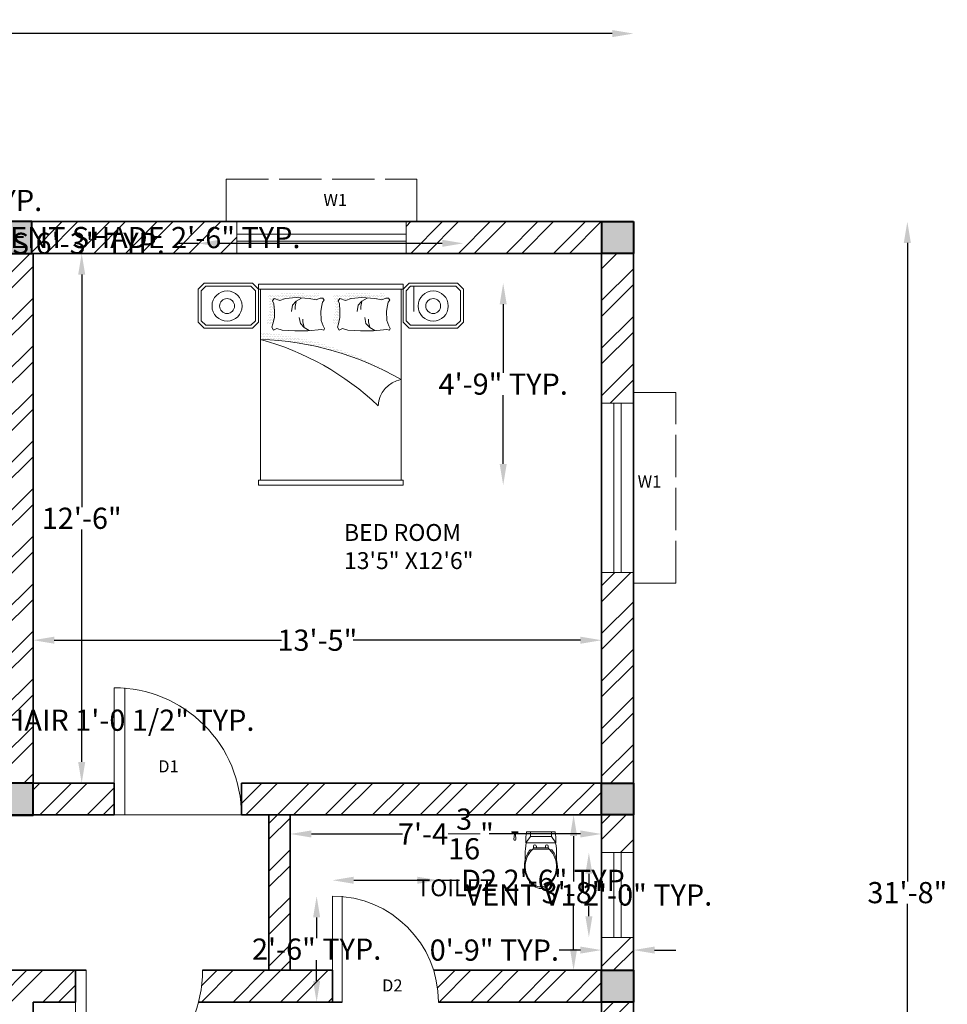
# Model space of a CAD drawing. Units: inches. Extents: x 3614 to 4242, y 2406 to 3033.
# Tile 10 of 10: x 3980 to 4242, y 2733 to 3012. Entities that reach past the tile are written whole.
import ezdxf

# ---------------------------------------------------------------- set-up
doc = ezdxf.new("R2010")
doc.units = ezdxf.units.IN
doc.linetypes.add('ACAD_ISO02W100', pattern=[15, 12, -3])
for name, color, linetype, lineweight in [('A-ANNO-DIMS', 2, 'Continuous', 18), ('A-ANNO-TEXT', 7, 'Continuous', 18), ('A-AREA-IDEN', 7, 'Continuous', 25), ('A-COLS', 7, 'Continuous', 40), ('A-COLS-PATT', 252, 'Continuous', 18), ('A-DOOR', 3, 'Continuous', 18), ('A-FLOR-FIXT', 9, 'Continuous', 18), ('A-FURN', 8, 'Continuous', 18), ('A-GLAZ', 4, 'Continuous', 18), ('A-GLAZ-OVHD', 8, 'ACAD_ISO02W100', 13), ('A-WALL', 7, 'Continuous', 35), ('A-WALL-PATT', 252, 'Continuous', 13)]:
    doc.layers.add(name, color=color, linetype=linetype, lineweight=lineweight)
doc.styles.get("Standard").update_dxf_attribs({"font": 'arial.ttf'})
doc.dimstyles.get("Standard").update_dxf_attribs({"dimtxt": 6, "dimasz": 6, "dimexe": 0.18, "dimexo": 0.0625, "dimgap": 0.09, "dimtad": 0, "dimtih": 1, "dimtoh": 1, "dimdec": 4, "dimzin": 0, "dimdsep": 46, "dimlunit": 4, "dimtxsty": 'Standard', "dimcen": 0.09, "dimse1": 1, "dimse2": 1, "dimadec": 0, "dimazin": 0, "dimtfac": 1, "dimtdec": 4, "dimtofl": 0, "dimtmove": 0, "dimatfit": 3, "dimfxl": 1, "dimtolj": 1, "dimtzin": 0, "dimarcsym": 0})
pattern_1 = [(270, (-3578.6833, 5895.14276), (0.451673685, -0.225836843), [0, -0.451673685])]

# ---------------------------------------------------------------- blocks, each defined once
blk = doc.blocks.new('*D8')
at = {"layer": 'A-ANNO-DIMS', "color": 0, "lineweight": -2, "transparency": 16777216}
for p, q in [((4136.4, 2780.34), (4136.4, 2767.5)), ((4136.4, 2748.34), (4136.4, 2761.19))]:
    blk.add_line(p, q, dxfattribs=at)
at = {"layer": 'A-ANNO-DIMS', "color": 0, "transparency": 16777216}
for points in [[(4135.4, 2780.34), (4137.4, 2780.34), (4136.4, 2786.34)], [(4135.4, 2748.34), (4137.4, 2748.34), (4136.4, 2742.34)]]:
    blk.add_solid(points, dxfattribs=at)
at = {"layer": 'Defpoints', "color": 0, "transparency": 16777216}
for p in [(4144.34, 2786.34), (4136.4, 2742.34), (4144.34, 2742.34)]:
    blk.add_point(p, dxfattribs=at)
at = {"layer": 'A-ANNO-DIMS', "color": 0, "transparency": 16777216, "insert": (4136.4, 2764.34), "char_height": 6, "attachment_point": 5}
blk.add_mtext('\\A1;3\'-8"', dxfattribs=at)
blk = doc.blocks.new('*D9')
at = {"layer": 'A-ANNO-DIMS', "color": 0, "lineweight": -2, "transparency": 16777216}
for p, q in [((4062.14, 2780.95), (4087.99, 2780.95)), ((4138.34, 2780.95), (4112.49, 2780.95))]:
    blk.add_line(p, q, dxfattribs=at)
at = {"layer": 'A-ANNO-DIMS', "color": 0, "transparency": 16777216}
for points in [[(4062.14, 2781.95), (4062.14, 2779.95), (4056.14, 2780.95)], [(4138.34, 2781.95), (4138.34, 2779.95), (4144.34, 2780.95)]]:
    blk.add_solid(points, dxfattribs=at)
at = {"layer": 'Defpoints', "color": 0, "transparency": 16777216}
for p in [(4056.14, 2786.34), (4144.34, 2786.34), (4144.34, 2780.95)]:
    blk.add_point(p, dxfattribs=at)
at = {"layer": 'A-ANNO-DIMS', "color": 0, "transparency": 16777216, "insert": (4100.24, 2780.95), "char_height": 6, "attachment_point": 5}
blk.add_mtext('\\A1;7\'-4{\\H1x;\\S3/16;}"', dxfattribs=at)
blk = doc.blocks.new('*D21')
at = {"layer": 'A-ANNO-DIMS', "color": 0, "lineweight": -2, "transparency": 16777216}
for p, q in [((3997.11, 2939.34), (3997.11, 2873.49)), ((3997.11, 2801.34), (3997.11, 2867.19))]:
    blk.add_line(p, q, dxfattribs=at)
at = {"layer": 'A-ANNO-DIMS', "color": 0, "transparency": 16777216}
for points in [[(3996.11, 2939.34), (3998.11, 2939.34), (3997.11, 2945.34)], [(3996.11, 2801.34), (3998.11, 2801.34), (3997.11, 2795.34)]]:
    blk.add_solid(points, dxfattribs=at)
at = {"layer": 'Defpoints', "color": 0, "transparency": 16777216}
for p in [(3992.71, 2945.34), (3992.71, 2795.34), (3997.11, 2795.34)]:
    blk.add_point(p, dxfattribs=at)
at = {"layer": 'A-ANNO-DIMS', "color": 0, "transparency": 16777216, "insert": (3997.11, 2870.34), "char_height": 6, "attachment_point": 5}
blk.add_mtext('\\A1;12\'-6"', dxfattribs=at)
blk = doc.blocks.new('*D22')
at = {"layer": 'A-ANNO-DIMS', "color": 0, "lineweight": -2, "transparency": 16777216}
for p, q in [((3989.34, 2835.82), (4053.72, 2835.82)), ((4138.34, 2835.82), (4073.95, 2835.82))]:
    blk.add_line(p, q, dxfattribs=at)
at = {"layer": 'A-ANNO-DIMS', "color": 0, "transparency": 16777216}
for points in [[(3989.34, 2836.82), (3989.34, 2834.82), (3983.34, 2835.82)], [(4138.34, 2836.82), (4138.34, 2834.82), (4144.34, 2835.82)]]:
    blk.add_solid(points, dxfattribs=at)
at = {"layer": 'Defpoints', "color": 0, "transparency": 16777216}
for p in [(3983.34, 2843.38), (4144.34, 2843.38), (4144.34, 2835.82)]:
    blk.add_point(p, dxfattribs=at)
at = {"layer": 'A-ANNO-DIMS', "color": 0, "transparency": 16777216, "insert": (4063.84, 2835.82), "char_height": 6, "attachment_point": 5}
blk.add_mtext('\\A1;13\'-5"', dxfattribs=at)
blk = doc.blocks.new('*D24')
at = {"layer": 'A-ANNO-DIMS', "color": 0, "lineweight": -2, "transparency": 16777216}
for p, q in [((3694.34, 3007.6), (3910.44, 3007.6)), ((4147.34, 3007.6), (3931.23, 3007.6))]:
    blk.add_line(p, q, dxfattribs=at)
at = {"layer": 'A-ANNO-DIMS', "color": 0, "transparency": 16777216}
for points in [[(3694.34, 3008.6), (3694.34, 3006.6), (3688.34, 3007.6)], [(4147.34, 3008.6), (4147.34, 3006.6), (4153.34, 3007.6)]]:
    blk.add_solid(points, dxfattribs=at)
at = {"layer": 'Defpoints', "color": 0, "transparency": 16777216}
for p in [(4153.34, 3007.6), (3688.34, 2954.34), (4153.34, 2954.34)]:
    blk.add_point(p, dxfattribs=at)
at = {"layer": 'A-ANNO-DIMS', "color": 0, "transparency": 16777216, "insert": (3920.84, 3007.6), "char_height": 6, "attachment_point": 5}
blk.add_mtext('\\A1;38\'-9"', dxfattribs=at)
blk = doc.blocks.new('*D25')
at = {"layer": 'A-ANNO-DIMS', "color": 0, "lineweight": -2, "transparency": 16777216}
for p, q in [((4230.92, 2948.34), (4230.92, 2767.5)), ((4230.92, 2580.34), (4230.92, 2761.19))]:
    blk.add_line(p, q, dxfattribs=at)
at = {"layer": 'A-ANNO-DIMS', "color": 0, "transparency": 16777216}
for points in [[(4229.92, 2948.34), (4231.92, 2948.34), (4230.92, 2954.34)], [(4229.92, 2580.34), (4231.92, 2580.34), (4230.92, 2574.34)]]:
    blk.add_solid(points, dxfattribs=at)
at = {"layer": 'Defpoints', "color": 0, "transparency": 16777216}
for p in [(4153.34, 2954.34), (4153.34, 2574.34), (4230.92, 2574.34)]:
    blk.add_point(p, dxfattribs=at)
at = {"layer": 'A-ANNO-DIMS', "color": 0, "transparency": 16777216, "insert": (4230.92, 2764.34), "char_height": 6, "attachment_point": 5}
blk.add_mtext('\\A1;31\'-8"', dxfattribs=at)
blk = doc.blocks.new('WINDOW-W1-48IN')
for p, q in [((48, 9), (0, 9)), ((0, 9), (0, 0)), ((48, 0), (48, 9)), ((0, 5.5), (48, 5.5)), ((0, 3.5), (48, 3.5)), ((0, 0), (48, 0))]:
    blk.add_line(p, q)
blk = doc.blocks.new('VENT-V1-24IN')
for p, q in [((24, 9), (0, 9)), ((0, 9), (0, 0)), ((24, 0), (24, 9)), ((0, 5.5), (24, 5.5)), ((0, 3.5), (24, 3.5)), ((0, 0), (24, 0))]:
    blk.add_line(p, q)
blk = doc.blocks.new('SHADE-W1')
for p, q in [((0, 0), (0, 12)), ((0, 12), (51, 12)), ((51, 12), (54, 12)), ((54, 12), (54, 0)), ((3, 0), (0, 0))]:
    blk.add_line(p, q)
blk = doc.blocks.new('COLUMN-9X9')
blk.add_lwpolyline([(9, 9), (0, 9), (0, 0), (9, 0)], close=True)
blk = doc.blocks.new('DOOR-SWING-30IN')
for p, q in [((0, 30), (0, 0)), ((2.75, 30), (2.75, 0)), ((0, 0), (2.75, 0))]:
    blk.add_line(p, q)
blk.add_arc((0, 0), 30, 0, 90)
blk = doc.blocks.new('DOOR-SWING-36IN')
for p, q in [((0, 36), (0, 0)), ((0, 0), (0, 36)), ((3, 0), (3, 36))]:
    blk.add_line(p, q)
blk.add_arc((0, 36), 36, 270, 0)
blk = doc.blocks.new('WC-PLAN')
for p, q in [((5.97, 11.16), (6.2, 11.58)), ((6.2, 11.58), (6.2, 12.03)), ((7.01, 11.58), (6.2, 11.58)), ((7.01, 12.03), (7.01, 11.58)), ((8.3, 11.58), (7.01, 11.58)), ((8.3, 11.58), (9.59, 11.58)), ((9.59, 12.03), (9.59, 11.58)), ((9.59, 11.58), (10.39, 11.58)), ((10.39, 11.58), (10.39, 12.03)), ((10.62, 11.16), (10.39, 11.58))]:
    blk.add_line(p, q)
for points in [[(1.85, 16.08), (0, 16.08)], [(1.73, 15.95), (0.11, 15.95)], [(1.35, 15.74), (0.5, 15.74)], [(0.5, 15.74), (0.5, 15.47), (0.8, 15.47)], [(0.72, 15.74), (0.72, 15.47)], [(0.8, 15.47), (1.07, 15.47)], [(1.07, 15.47), (1.34, 15.47), (1.35, 15.74)], [(1.15, 15.74), (1.15, 15.47)], [(4.05, 12.98), (5.32, 14.75), (5.32, 16.08)], [(12.37, 16.08), (4.22, 16.08)], [(5.32, 14.75), (8.3, 14.75)], [(11.28, 14.75), (8.3, 14.75)], [(12.54, 12.98), (11.28, 14.75), (11.28, 16.08)], [(4.13, 12.98), (8.3, 12.98)], [(12.47, 12.98), (8.3, 12.98)]]:
    blk.add_lwpolyline(points)
for points in [[(0.5, 15.74, -0.158381), (0, 16.08, 2.932383)], [(0.8, 15.45), (0.63, 13.98, 0.482607), (0.95, 13.67, -0.547905)], [(1.07, 15.45), (1.23, 13.98, -0.482607), (0.92, 13.67, 0.547905)], [(1.35, 15.74, 0.158381), (1.85, 16.08, -2.932383)], [(4.22, 16.08, 0.056711), (4.05, 12.98), (4.13, 12.98)], [(12.37, 16.08, -0.056711), (12.54, 12.98), (12.47, 12.98)], [(4.13, 12.98, 0.052121), (3.84, 9.61), (3.84, 8.13, 0.14456)], [(5.97, 11.16, 0.008985), (5.8, 11, 0.182634)], [(8.3, 11.16), (5.97, 11.16, 0.008985)], [(8.3, 11.16), (10.62, 11.16, -0.444938)], [(10.62, 11.16, -0.008985), (10.79, 11, -0.182634)], [(12.47, 12.98, -0.052121), (12.76, 9.61), (12.76, 8.13, -0.14456)], [(5.24, 11, 0.11024), (3.84, 8.13, 0.16845)], [(5.8, 11, 0.434217), (6.2, 1.23, 0.182634), (8.3, 0.47, 2.693815)], [(5.8, 11), (5.24, 11, 0.416606)], [(10.79, 11, -0.434217), (10.39, 1.23, -0.182634), (8.3, 0.47, -2.693815)], [(10.79, 11), (11.35, 11, -0.416606)], [(11.35, 11, -0.11024), (12.76, 8.13, -0.16845)], [(3.84, 8.13, 0.292914), (6.42, 0.65, 0.16845), (8.3, 0, 2.883082)], [(12.76, 8.13, -0.292914), (10.17, 0.65, -0.16845), (8.3, 0, -2.883082)]]:
    blk.add_lwpolyline(points, format="xyb")
for centre in [(6.6, 12.03), (9.99, 12.03)]:
    blk.add_arc(centre, 0.403, 0, 180)
blk = doc.blocks.new('BED-DOUBLE-WITH-NIGHTSTANDS')
h = blk.add_hatch()
h.set_pattern_fill('DOTS', color=256, scale=0.284519, angle=-90, style=0)
h.set_pattern_definition(pattern_1)
h.paths.add_polyline_path([(43.21, 57.47), (41.26, 57.47, -0.124273), (29.87, 17.64, 0.122563)])
h = blk.add_hatch()
h.set_pattern_fill('DOTS', color=256, scale=0.284519, angle=-90, style=0)
h.set_pattern_definition(pattern_1)
h.paths.add_polyline_path([(53.82, 40.86), (54.34, 41.21), (54.34, 42), (53.9, 43.14), (54.25, 45.06), (54.52, 48.74), (54.25, 51.8), (53.73, 53.38), (54.25, 55.04), (53.55, 55.48), (52.77, 55.13), (50.75, 54.95), (48.83, 54.95), (47.08, 55.39), (46.12, 55.65), (45.33, 55.22), (45.77, 54.25), (45.69, 53.96), (47.41, 53.53), (49.34, 53.53), (51.35, 53.71), (52.13, 54.06), (52.83, 53.62), (52.31, 51.96), (52.83, 50.38), (53.1, 47.32), (52.83, 43.64), (52.48, 41.72), (52.6, 41.41), (53.2, 41.3)])
h.paths.add_polyline_path([(53.82, 22.27), (54.34, 22.62), (54.34, 23.41), (53.9, 24.55), (54.25, 26.48), (54.52, 30.15), (54.25, 33.21), (53.73, 34.79), (54.25, 36.45), (53.55, 36.89), (52.77, 36.54), (50.75, 36.37), (48.83, 36.37), (47.08, 36.8), (46.12, 37.07), (45.33, 36.63), (45.77, 35.67), (45.69, 35.38), (47.41, 34.95), (49.34, 34.95), (51.35, 35.12), (52.13, 35.47), (52.83, 35.03), (52.31, 33.37), (52.83, 31.79), (53.1, 28.73), (52.83, 25.05), (52.48, 23.13), (52.6, 22.82), (53.2, 22.71)])
for p, q in [((0, 17.07), (0, 58.04)), ((0, 58.04), (1.42, 58.04)), ((1.42, 17.07), (1.42, 58.04)), ((1.42, 57.47), (55.48, 57.47)), ((55.48, 17.07), (55.48, 58.04)), ((55.48, 58.04), (56.9, 58.04)), ((56.9, 17.07), (56.9, 58.04)), ((1.42, 17.07), (0, 17.07)), ((55.48, 17.64), (1.42, 17.64)), ((56.9, 17.07), (55.48, 17.07)), ((56.3, 14.01), (49.19, 14.01))]:
    blk.add_line(p, q)
for points in [[(44.39, 73.41), (44.39, 59.75), (46.09, 58.04), (55.48, 58.04), (57.19, 59.75), (57.19, 73.41), (55.48, 75.11), (46.09, 75.11)], [(45.24, 72.98), (45.24, 60.18), (46.52, 58.9), (55.05, 58.9), (56.33, 60.18), (56.33, 72.98), (55.05, 74.26), (46.52, 74.26)], [(44.39, 15.36), (44.39, 1.71), (46.09, 0), (55.48, 0), (57.19, 1.71), (57.19, 15.36), (55.48, 17.07), (46.09, 17.07)], [(45.24, 14.94), (45.24, 2.13), (46.52, 0.85), (55.05, 0.85), (56.33, 2.13), (56.33, 14.94), (55.05, 16.22), (46.52, 16.22)]]:
    blk.add_lwpolyline(points, close=True)
for points in [[(52.31, 51.96), (52.83, 53.62), (52.13, 54.06), (51.35, 53.71), (49.34, 53.53), (47.41, 53.53), (45.66, 53.97), (44.7, 54.23), (43.91, 53.8), (44.35, 52.83), (43.91, 51.34), (43.65, 47.76), (43.65, 44.08), (44.09, 40.23), (43.91, 39.53), (44.35, 39.35), (45.05, 39.7), (46.62, 40.32), (49.25, 40.4), (50.82, 40.05), (51.78, 39.88), (52.4, 39.44), (52.92, 39.79), (52.92, 40.58), (52.48, 41.72), (52.83, 43.64), (53.1, 47.32), (52.83, 50.38), (52.31, 51.96)], [(52.92, 45.83), (52.05, 47.32), (50.91, 48.37), (49.16, 48.72)], [(51.96, 47.32), (50.56, 47.67), (49.69, 47.67)], [(43.74, 43.64), (44.61, 45.13), (45.75, 46.18), (47.5, 46.53)], [(44.7, 45.13), (46.1, 45.48), (46.97, 45.48)], [(52.31, 33.37), (52.83, 35.03), (52.13, 35.47), (51.35, 35.12), (49.34, 34.95), (47.41, 34.95), (45.66, 35.38), (44.7, 35.65), (43.91, 35.21), (44.35, 34.24), (43.91, 32.76), (43.65, 29.17), (43.65, 25.49), (44.09, 21.64), (43.91, 20.94), (44.35, 20.77), (45.05, 21.12), (46.62, 21.73), (49.25, 21.82), (50.82, 21.47), (51.78, 21.29), (52.4, 20.85), (52.92, 21.2), (52.92, 21.99), (52.48, 23.13), (52.83, 25.05), (53.1, 28.73), (52.83, 31.79), (52.31, 33.37)], [(43.74, 25.05), (44.61, 26.54), (45.75, 27.59), (47.5, 27.94)], [(52.92, 27.24), (52.05, 28.73), (50.91, 29.78), (49.16, 30.13)], [(51.96, 28.73), (50.56, 29.08), (49.69, 29.08)], [(44.7, 26.54), (46.1, 26.89), (46.97, 26.89)]]:
    blk.add_lwpolyline(points)
for centre, radius in [((50.7, 66.92), 4.27), ((50.7, 66.92), 2.11), ((50.7, 8.56), 4.27), ((50.7, 8.56), 2.11)]:
    blk.add_circle(centre, radius)
for centre, radius, start, end in [((-34.21, 78.09), 78.23, 316.4367, 344.7234), ((-43.33, 60.1), 84.62, 329.8866, 358.2226), ((22.03, 16.21), 7.98, 10.3543, 86.7862)]:
    blk.add_arc(centre, radius, start, end)
blk = doc.blocks.new('*D45')
at = {"layer": 'A-ANNO-DIMS', "color": 0, "lineweight": -2, "transparency": 16777216}
for p, q in [((3931.73, 2825.5), (3931.73, 2825.16)), ((3931.73, 2819.16), (3931.73, 2813.16)), ((3931.73, 2813.16), (3937.73, 2813.16))]:
    blk.add_line(p, q, dxfattribs=at)
at = {"layer": 'A-ANNO-DIMS', "color": 0, "transparency": 16777216}
for points in [[(3932.73, 2825.5), (3930.73, 2825.5), (3931.73, 2831.5)], [(3932.73, 2825.16), (3930.73, 2825.16), (3931.73, 2819.16)]]:
    blk.add_solid(points, dxfattribs=at)
at = {"layer": 'Defpoints', "color": 0, "transparency": 16777216}
for p in [(3933.58, 2831.5), (3931.73, 2819.16), (3933.58, 2819.16)]:
    blk.add_point(p, dxfattribs=at)
at = {"layer": 'A-ANNO-DIMS', "color": 0, "transparency": 16777216, "insert": (3992.99, 2813.16), "char_height": 6, "attachment_point": 5}
blk.add_mtext('\\A1;DINING CHAIR 1\'-0 1/2" TYP.', dxfattribs=at)
blk = doc.blocks.new('*D47')
at = {"layer": 'A-ANNO-DIMS', "color": 0, "lineweight": -2, "transparency": 16777216}
for p, q in [((4140.74, 2769.67), (4140.74, 2766.82)), ((4140.74, 2757.67), (4140.74, 2760.51))]:
    blk.add_line(p, q, dxfattribs=at)
at = {"layer": 'A-ANNO-DIMS', "color": 0, "transparency": 16777216}
for points in [[(4139.74, 2769.67), (4141.74, 2769.67), (4140.74, 2775.67)], [(4139.74, 2757.67), (4141.74, 2757.67), (4140.74, 2751.67)]]:
    blk.add_solid(points, dxfattribs=at)
at = {"layer": 'Defpoints', "color": 0, "transparency": 16777216}
for p in [(4140.74, 2775.67), (4144.34, 2775.67), (4144.34, 2751.67)]:
    blk.add_point(p, dxfattribs=at)
at = {"layer": 'A-ANNO-DIMS', "color": 0, "transparency": 16777216, "insert": (4140.74, 2763.67), "char_height": 6, "attachment_point": 5}
blk.add_mtext('\\A1;VENT V1 2\'-0" TYP.', dxfattribs=at)
blk = doc.blocks.new('*D48')
at = {"layer": 'A-ANNO-DIMS', "color": 0, "lineweight": -2, "transparency": 16777216}
for p, q in [((4138.34, 2748.07), (4132.34, 2748.07)), ((4159.34, 2748.07), (4165.34, 2748.07))]:
    blk.add_line(p, q, dxfattribs=at)
at = {"layer": 'A-ANNO-DIMS', "color": 0, "transparency": 16777216}
for points in [[(4138.34, 2749.07), (4138.34, 2747.07), (4144.34, 2748.07)], [(4159.34, 2749.07), (4159.34, 2747.07), (4153.34, 2748.07)]]:
    blk.add_solid(points, dxfattribs=at)
at = {"layer": 'Defpoints', "color": 0, "transparency": 16777216}
for p in [(4144.34, 2751.67), (4153.34, 2751.67), (4144.34, 2748.07)]:
    blk.add_point(p, dxfattribs=at)
at = {"layer": 'A-ANNO-DIMS', "color": 0, "transparency": 16777216, "insert": (4113.96, 2748.07), "char_height": 6, "attachment_point": 5}
blk.add_mtext('\\A1;0\'-9" TYP.', dxfattribs=at)
blk = doc.blocks.new('*D51')
at = {"layer": 'A-ANNO-DIMS', "color": 0, "lineweight": -2, "transparency": 16777216}
for p, q in [((3939.12, 2949.84), (3957.12, 2949.84)), ((3963.12, 2949.84), (3969.12, 2949.84))]:
    blk.add_line(p, q, dxfattribs=at)
at = {"layer": 'A-ANNO-DIMS', "color": 0, "transparency": 16777216}
for points in [[(3939.12, 2950.84), (3939.12, 2948.84), (3933.12, 2949.84)], [(3957.12, 2950.84), (3957.12, 2948.84), (3963.12, 2949.84)]]:
    blk.add_solid(points, dxfattribs=at)
at = {"layer": 'Defpoints', "color": 0, "transparency": 16777216}
for p in [(3933.12, 2954.34), (3963.12, 2954.34), (3963.12, 2949.84)]:
    blk.add_point(p, dxfattribs=at)
at = {"layer": 'A-ANNO-DIMS', "color": 0, "transparency": 16777216, "insert": (4015.6, 2949.84), "char_height": 6, "attachment_point": 5}
blk.add_mtext('\\A1;VENT SHADE 2\'-6" TYP.', dxfattribs=at)
blk = doc.blocks.new('*D52')
at = {"layer": 'A-ANNO-DIMS', "color": 0, "lineweight": -2, "transparency": 16777216}
for p, q in [((3967.62, 2972.34), (3967.62, 2978.34)), ((3967.62, 2948.34), (3967.62, 2942.34))]:
    blk.add_line(p, q, dxfattribs=at)
at = {"layer": 'A-ANNO-DIMS', "color": 0, "transparency": 16777216}
for points in [[(3966.62, 2972.34), (3968.62, 2972.34), (3967.62, 2966.34)], [(3966.62, 2948.34), (3968.62, 2948.34), (3967.62, 2954.34)]]:
    blk.add_solid(points, dxfattribs=at)
at = {"layer": 'Defpoints', "color": 0, "transparency": 16777216}
for p in [(3963.12, 2966.34), (3967.62, 2966.34), (3963.12, 2954.34)]:
    blk.add_point(p, dxfattribs=at)
at = {"layer": 'A-ANNO-DIMS', "color": 0, "transparency": 16777216, "insert": (3967.62, 2960.34), "char_height": 6, "attachment_point": 5}
blk.add_mtext('\\A1;1\'-0" TYP.', dxfattribs=at)
blk = doc.blocks.new('*D53')
at = {"layer": 'A-ANNO-DIMS', "color": 0, "lineweight": -2, "transparency": 16777216}
for p, q in [((4074.14, 2767.84), (4092.14, 2767.84)), ((4098.14, 2767.84), (4104.14, 2767.84))]:
    blk.add_line(p, q, dxfattribs=at)
at = {"layer": 'A-ANNO-DIMS', "color": 0, "transparency": 16777216}
for points in [[(4074.14, 2768.84), (4074.14, 2766.84), (4068.14, 2767.84)], [(4092.14, 2768.84), (4092.14, 2766.84), (4098.14, 2767.84)]]:
    blk.add_solid(points, dxfattribs=at)
at = {"layer": 'Defpoints', "color": 0, "transparency": 16777216}
for p in [(4098.14, 2767.84), (4068.14, 2763.34), (4098.14, 2763.34)]:
    blk.add_point(p, dxfattribs=at)
at = {"layer": 'A-ANNO-DIMS', "color": 0, "transparency": 16777216, "insert": (4128.89, 2767.84), "char_height": 6, "attachment_point": 5}
blk.add_mtext('\\A1;D2 2\'-6" TYP.', dxfattribs=at)
blk = doc.blocks.new('*D54')
at = {"layer": 'A-ANNO-DIMS', "color": 0, "lineweight": -2, "transparency": 16777216}
for p, q in [((4063.64, 2757.34), (4063.64, 2751.49)), ((4063.64, 2739.34), (4063.64, 2745.19))]:
    blk.add_line(p, q, dxfattribs=at)
at = {"layer": 'A-ANNO-DIMS', "color": 0, "transparency": 16777216}
for points in [[(4062.64, 2757.34), (4064.64, 2757.34), (4063.64, 2763.34)], [(4062.64, 2739.34), (4064.64, 2739.34), (4063.64, 2733.34)]]:
    blk.add_solid(points, dxfattribs=at)
at = {"layer": 'Defpoints', "color": 0, "transparency": 16777216}
for p in [(4063.64, 2763.34), (4068.14, 2763.34), (4068.14, 2733.34)]:
    blk.add_point(p, dxfattribs=at)
at = {"layer": 'A-ANNO-DIMS', "color": 0, "transparency": 16777216, "insert": (4063.64, 2748.34), "char_height": 6, "attachment_point": 5}
blk.add_mtext('\\A1;2\'-6" TYP.', dxfattribs=at)
blk = doc.blocks.new('*D57')
at = {"layer": 'A-ANNO-DIMS', "color": 0, "lineweight": -2, "transparency": 16777216}
for p, q in [((4030.09, 2948.2), (4024.09, 2948.2)), ((4099.2, 2948.2), (4036.09, 2948.2))]:
    blk.add_line(p, q, dxfattribs=at)
at = {"layer": 'A-ANNO-DIMS', "color": 0, "transparency": 16777216}
for points in [[(4036.09, 2949.2), (4036.09, 2947.2), (4030.09, 2948.2)], [(4099.2, 2949.2), (4099.2, 2947.2), (4105.2, 2948.2)]]:
    blk.add_solid(points, dxfattribs=at)
at = {"layer": 'Defpoints', "color": 0, "transparency": 16777216}
for p in [(4030.09, 2948.2), (4030.09, 2936.94), (4105.2, 2936.94)]:
    blk.add_point(p, dxfattribs=at)
at = {"layer": 'A-ANNO-DIMS', "color": 0, "transparency": 16777216, "insert": (3960.9, 2948.2), "char_height": 6, "attachment_point": 5}
blk.add_mtext('\\A1;BED & NIGHTSTANDS 6\'-3" TYP.', dxfattribs=at)
blk = doc.blocks.new('*D58')
at = {"layer": 'A-ANNO-DIMS', "color": 0, "lineweight": -2, "transparency": 16777216}
for p, q in [((4116.47, 2930.94), (4116.47, 2911.49)), ((4116.47, 2885.75), (4116.47, 2905.19))]:
    blk.add_line(p, q, dxfattribs=at)
at = {"layer": 'A-ANNO-DIMS', "color": 0, "transparency": 16777216}
for points in [[(4115.47, 2930.94), (4117.47, 2930.94), (4116.47, 2936.94)], [(4115.47, 2885.75), (4117.47, 2885.75), (4116.47, 2879.75)]]:
    blk.add_solid(points, dxfattribs=at)
at = {"layer": 'Defpoints', "color": 0, "transparency": 16777216}
for p in [(4105.2, 2936.94), (4116.47, 2936.94), (4105.2, 2879.75)]:
    blk.add_point(p, dxfattribs=at)
at = {"layer": 'A-ANNO-DIMS', "color": 0, "transparency": 16777216, "insert": (4116.47, 2908.34), "char_height": 6, "attachment_point": 5}
blk.add_mtext('\\A1;4\'-9" TYP.', dxfattribs=at)

msp = doc.modelspace()

# ---------------------------------------------------------------- hatches: boundary and pattern name
at = {"layer": 'A-COLS-PATT'}
h = msp.add_hatch(color=256, dxfattribs=at)
h.dxf.hatch_style = 1
h.paths.add_polyline_path([(3697.336, 2954.34049), (3688.336, 2954.34049), (3688.336, 2945.34049), (3697.336, 2945.34049)])
h.paths.add_polyline_path([(3818.336, 2954.34049), (3809.336, 2954.34049), (3809.336, 2945.34049), (3818.336, 2945.34049)])
h.paths.add_polyline_path([(3818.336, 2787.28572), (3809.336, 2787.28572), (3809.336, 2778.34049), (3818.336, 2778.34049)])
h.paths.add_polyline_path([(3697.336, 2742.34049), (3688.336, 2742.34049), (3688.336, 2733.34049), (3697.336, 2733.34049)])
h.paths.add_polyline_path([(3697.336, 2583.37355), (3688.336, 2583.37355), (3688.336, 2574.37355), (3697.336, 2574.37355)])
h.paths.add_polyline_path([(3899.336, 2583.34049), (3890.336, 2583.34049), (3890.336, 2574.34049), (3899.336, 2574.34049)])
h.paths.add_polyline_path([(3983.336, 2583.34049), (3974.336, 2583.34049), (3974.336, 2574.34049), (3983.336, 2574.34049)])
h.paths.add_polyline_path([(4153.336, 2583.34049), (4144.336, 2583.34049), (4144.336, 2574.34049), (4153.336, 2574.34049)])
h.paths.add_polyline_path([(4153.336, 2742.34049), (4144.336, 2742.34049), (4144.336, 2733.34049), (4153.336, 2733.34049)])
h.paths.add_polyline_path([(4153.336, 2795.34049), (4144.336, 2795.34049), (4144.336, 2786.34049), (4153.336, 2786.34049)])
h.paths.add_polyline_path([(3983.336, 2795.31105), (3974.336, 2795.31105), (3974.336, 2786.34049), (3983.336, 2786.34049)])
h.paths.add_polyline_path([(4153.336, 2954.34049), (4144.36882, 2954.34049), (4144.36882, 2945.34049), (4153.336, 2945.34049)])
h.paths.add_polyline_path([(3982.96188, 2954.34049), (3973.96188, 2954.34049), (3973.96188, 2945.34049), (3982.96188, 2945.34049)])
at = {"layer": 'A-WALL-PATT'}
h = msp.add_hatch(dxfattribs=at)
h.set_pattern_fill('ANSI32', color=256)
h.paths.add_polyline_path([(4041.01458, 2954.34049), (3982.96188, 2954.34049), (3982.96188, 2945.34049), (3983.336, 2945.34049), (4041.01458, 2945.34049)])
h.paths.add_polyline_path([(3973.96188, 2954.34049), (3960.11861, 2954.34049), (3960.11861, 2945.34049), (3973.96188, 2945.34049)])
h.paths.add_polyline_path([(3936.11861, 2954.34049), (3901.17016, 2954.34049), (3901.17016, 2945.34049), (3913.336, 2945.34049), (3913.336, 2896.34049, -0.050382044), (3919.336, 2895.73437), (3919.336, 2945.34049), (3936.11861, 2945.34049)])
h.paths.add_polyline_path([(3983.336, 2945.34049), (3982.96188, 2945.34049), (3974.336, 2945.34049), (3974.336, 2873.34049), (3974.336, 2795.31105), (3983.336, 2795.31105), (3983.336, 2867.34049)])
h.paths.add_polyline_path([(3974.336, 2872.34049), (3919.336, 2872.34049), (3858.336, 2872.34049), (3858.336, 2866.34049), (3919.336, 2866.34049), (3974.336, 2866.34049)])
h.paths.add_polyline_path([(3877.17016, 2954.34049), (3852.34021, 2954.34049), (3852.34021, 2945.34049), (3852.336, 2896.34049), (3858.336, 2896.34049), (3858.336, 2945.34049), (3877.17016, 2945.34049)])
h.paths.add_polyline_path([(3871.94212, 2902.34049), (3858.336, 2902.34049), (3858.336, 2896.34049), (3871.336, 2896.34049, -0.050382044)], flags=0)
h.paths.add_polyline_path([(3913.336, 2902.34049), (3901.336, 2902.34049), (3901.336, 2896.34049), (3913.336, 2896.34049)], flags=17)
h.paths.add_polyline_path([(3858.336, 2872.34049), (3852.336, 2872.34049), (3852.336, 2866.34049), (3858.336, 2866.34049)])
h.paths.add_polyline_path([(3809.336, 2954.34049), (3764.4617, 2954.34049), (3764.4617, 2945.34049), (3809.336, 2945.34049)])
h.paths.add_polyline_path([(3716.4617, 2954.34049), (3697.336, 2954.34049), (3697.336, 2945.34049), (3716.4617, 2945.34049)])
h.paths.add_polyline_path([(3697.336, 2945.34049), (3688.336, 2945.34049), (3688.336, 2894.73438), (3697.336, 2894.73438)])
h = msp.add_hatch(dxfattribs=at)
h.set_pattern_fill('ANSI32', color=256)
h.paths.add_polyline_path([(4153.336, 2945.34049), (4144.336, 2945.34049), (4144.336, 2902.95478), (4153.336, 2902.95478)])
h.paths.add_polyline_path([(4144.36882, 2954.34049), (4089.01458, 2954.34049), (4089.01458, 2945.34049), (4144.36882, 2945.34049)])
h.paths.add_polyline_path([(3818.336, 2945.34049), (3809.336, 2945.34049), (3809.336, 2787.28572), (3818.336, 2787.28572)])
h.paths.add_polyline_path([(3697.336, 2846.73438), (3688.336, 2846.73438), (3688.336, 2742.34049), (3697.336, 2742.34049)])
h.paths.add_polyline_path([(3854.336, 2742.34049), (3853.36389, 2742.34049), (3818.336, 2742.34049), (3809.336, 2742.34049), (3697.336, 2742.34049), (3697.336, 2733.34049), (3809.336, 2733.34049), (3854.336, 2733.34049)])
h.paths.add_polyline_path([(3697.336, 2733.34049), (3688.336, 2733.34049), (3688.336, 2690.05693), (3697.336, 2690.05693)])
h.paths.add_polyline_path([(3697.336, 2642.05693), (3688.336, 2642.05693), (3688.336, 2583.37355), (3697.336, 2583.37355)])
h.paths.add_polyline_path([(3726.39802, 2583.34049), (3697.336, 2583.34049), (3697.336, 2574.34049), (3726.39802, 2574.34049)])
h.paths.add_polyline_path([(3842.336, 2583.34049), (3818.336, 2583.34049), (3809.336, 2583.34049), (3774.39802, 2583.34049), (3774.39802, 2574.34049), (3809.336, 2574.34049), (3842.336, 2574.34049)])
h.paths.add_polyline_path([(3890.336, 2583.34049), (3878.336, 2583.34049), (3878.336, 2574.34049), (3890.336, 2574.34049)])
h = msp.add_hatch(dxfattribs=at)
h.set_pattern_fill('ANSI32', color=256)
h.paths.add_polyline_path([(3899.336, 2733.34049), (3899.336, 2742.34049), (3890.336, 2742.34049), (3890.336, 2583.34049), (3899.336, 2583.34049)])
h.paths.add_polyline_path([(3983.336, 2733.34049), (3995.336, 2733.34049), (3995.336, 2742.34049), (3983.336, 2742.34049), (3974.336, 2742.34049), (3974.336, 2583.34049), (3983.336, 2583.34049)])
h.paths.add_polyline_path([(3974.336, 2583.34049), (3899.336, 2583.34049), (3899.336, 2574.34049), (3974.336, 2574.34049)])
h.paths.add_polyline_path([(4045.73114, 2583.34049), (3983.336, 2583.34049), (3983.336, 2574.34049), (4045.73114, 2574.34049)])
h.paths.add_polyline_path([(4144.336, 2583.34049), (4093.73114, 2583.34049), (4093.73114, 2574.34049), (4144.336, 2574.34049)])
h.paths.add_polyline_path([(4153.336, 2639.00845), (4144.336, 2639.00845), (4144.336, 2583.34049), (4153.336, 2583.34049)])
h.paths.add_polyline_path([(4153.336, 2733.34049), (4144.336, 2733.34049), (4144.336, 2687.00845), (4153.336, 2687.00845)])
h.paths.add_polyline_path([(4144.336, 2742.34049), (4096.76112, 2742.34049, -0.076320834), (4098.14294, 2733.34049), (4144.336, 2733.34049)])
h.paths.add_polyline_path([(4068.14294, 2742.34049), (4056.14294, 2742.34049), (4031.336, 2742.34049, -0.063254224), (4030.19285, 2733.34049), (4068.14294, 2733.34049)])
h.paths.add_polyline_path([(4144.336, 2795.34049), (4042.336, 2795.34049), (4042.336, 2786.34049), (4144.336, 2786.34049)])
h.paths.add_polyline_path([(4153.336, 2854.95478), (4144.336, 2854.95478), (4144.336, 2795.34049), (4153.336, 2795.34049)])
h = msp.add_hatch(dxfattribs=at)
h.set_pattern_fill('ANSI32', color=256)
h.paths.add_polyline_path([(4006.336, 2795.34049), (3983.336, 2795.34049), (3983.336, 2786.34049), (4006.336, 2786.34049)])
h = msp.add_hatch(dxfattribs=at)
h.set_pattern_fill('ANSI32', color=256)
h.paths.add_polyline_path([(4056.14294, 2786.34049), (4050.14294, 2786.34049), (4050.14294, 2742.34049), (4056.14294, 2742.34049)])
h = msp.add_hatch(dxfattribs=at)
h.set_pattern_fill('ANSI32', color=256)
h.paths.add_polyline_path([(4153.336, 2786.34049), (4144.336, 2786.34049), (4144.336, 2775.6675), (4153.336, 2775.6675)])
h.paths.add_polyline_path([(4153.336, 2751.6675), (4144.336, 2751.6675), (4144.336, 2742.34049), (4153.336, 2742.34049)])

# ---------------------------------------------------------------- linework, layer by layer
at = {"layer": 'A-DOOR'}
for p, q in [((4006.336, 2786.34049), (4042.336, 2786.34049)), ((3995.336, 2742.34049), (3998.336, 2742.34049))]:
    msp.add_line(p, q, dxfattribs=at)
at = {"layer": 'A-GLAZ-OVHD'}
for p, q in [((4165.36739, 2905.95478), (4153.336, 2905.95478)), ((4165.36739, 2902.95478), (4165.36739, 2905.95478)), ((4165.36739, 2851.95494), (4165.36739, 2902.95478)), ((4153.336, 2854.95478), (4153.36739, 2851.95494)), ((4153.36739, 2851.95494), (4165.36739, 2851.95494))]:
    msp.add_line(p, q, dxfattribs=at)
at = {"layer": 'A-WALL'}
for p, q in [((3852.34021, 2954.34049), (4153.336, 2954.34049)), ((4153.336, 2954.34049), (4153.336, 2574.34049)), ((3982.96188, 2945.34049), (3983.336, 2945.34049)), ((3983.336, 2945.34049), (3983.336, 2867.34049)), ((3983.336, 2945.34049), (4144.336, 2945.34049)), ((4144.336, 2945.34049), (4144.336, 2795.34049)), ((3983.336, 2795.34049), (3983.336, 2867.34049)), ((3983.336, 2795.34049), (4006.336, 2795.34049)), ((4006.336, 2795.34049), (4006.336, 2786.34049)), ((4042.336, 2786.34049), (4042.336, 2795.34049)), ((4042.336, 2795.34049), (4144.336, 2795.34049)), ((3974.336, 2786.34049), (3983.336, 2786.34049)), ((3983.336, 2786.34049), (4006.336, 2786.34049)), ((4042.336, 2786.34049), (4144.336, 2786.34049)), ((4050.14294, 2786.34049), (4050.14294, 2742.34049)), ((4056.14294, 2786.34049), (4056.14294, 2742.34049)), ((4144.336, 2786.34049), (4144.336, 2742.34049)), ((3974.336, 2742.34049), (3983.336, 2742.34049)), ((3998.336, 2742.34049), (3983.336, 2742.34049)), ((3995.336, 2733.34049), (3995.336, 2742.34049)), ((4068.14294, 2742.34049), (4031.336, 2742.34049)), ((4056.14294, 2742.34049), (4068.14294, 2742.34049)), ((4068.14294, 2742.34049), (4068.14294, 2733.34049)), ((4144.336, 2742.34049), (4096.76112, 2742.34049)), ((3983.336, 2733.34049), (3983.336, 2583.34049)), ((3983.336, 2733.34049), (3995.336, 2733.34049)), ((3995.336, 2733.34049), (3983.336, 2733.34049)), ((3995.336, 2733.34049), (3983.336, 2733.34049)), ((4070.89294, 2733.34049), (4030.19285, 2733.34049)), ((4070.89294, 2733.34049), (4030.19285, 2733.34049)), ((4098.14294, 2733.34049), (4144.336, 2733.34049)), ((4144.336, 2733.34049), (4144.336, 2583.34049))]:
    msp.add_line(p, q, dxfattribs=at)

# ---------------------------------------------------------------- block references
at = {"layer": 'A-COLS'}
for p in [(3973.96188, 2945.34), (3974.336, 2786.31056)]:
    msp.add_blockref('COLUMN-9X9', p, dxfattribs=at)
at = {"layer": 'A-COLS', "extrusion": (0, 0, -1), "zscale": -1, "rotation": 89.99999999999999}
for p in [(-4144.36833, 2945.34049), (-4144.33551, 2786.34049), (-4144.33551, 2733.34049)]:
    msp.add_blockref('COLUMN-9X9', p, dxfattribs=at)
at = {"layer": 'A-DOOR', "extrusion": (0, 0, -1), "zscale": -1, "rotation": 180}
msp.add_blockref('DOOR-SWING-36IN', (-4006.336, 2822.34099), dxfattribs=at)
at = {"layer": 'A-DOOR'}
for name, p in [('DOOR-SWING-30IN', (4068.143, 2733.34)), ('DOOR-SWING-36IN', (3995.336, 2706.34))]:
    msp.add_blockref(name, p, dxfattribs=at)
at = {"layer": 'A-FLOR-FIXT'}
msp.add_blockref('WC-PLAN', (4118.84961, 2765.48455), dxfattribs=at)
at = {"layer": 'A-FURN', "rotation": 90.0000000000044}
msp.add_blockref('BED-DOUBLE-WITH-NIGHTSTANDS', (4105.20387, 2879.74692), dxfattribs=at)
at = {"layer": 'A-GLAZ', "extrusion": (0, 0, -1), "zscale": -1}
for p, rotation in [((-4041.01488, 2954.34099), 180), ((-4144.33551, 2854.95508), 90.00000000000003)]:
    msp.add_blockref('WINDOW-W1-48IN', p, dxfattribs=dict(at, rotation=rotation))
at = {"layer": 'A-GLAZ', "rotation": 90.00000000000047}
msp.add_blockref('VENT-V1-24IN', (4153.33649, 2751.66788), dxfattribs=at)
at = {"layer": 'A-GLAZ-OVHD'}
msp.add_blockref('SHADE-W1', (4038.01488, 2954.34), dxfattribs=at)

# ---------------------------------------------------------------- texts
at = {"layer": 'A-ANNO-TEXT', "char_height": 3.42604, "attachment_point": 1}
for s, insert in [('W1', (4065.57297, 2962.18652)), ('W1', (4154.54639, 2882.46485)), ('D1', (4018.76443, 2801.81514)), ('D2', (4082.1534, 2739.77214))]:
    msp.add_mtext_dynamic_manual_height_columns(s, width=192.8287007, gutter_width=17.1302, heights=[0], dxfattribs=dict(at, insert=insert))
at = {"layer": 'A-AREA-IDEN', "attachment_point": 1}
for s, width, gutter_width, insert, char_height in [('BED ROOM\\P13\'5" X12\'6"', 126.6171413, 23.88852, (4071.37864, 2868.71308), 4.7777047), ('TOILET', 66.2541682, 12.5, (4091.89796, 2768.09519), 4.777705)]:
    msp.add_mtext_dynamic_manual_height_columns(s, width=width, gutter_width=gutter_width, heights=[0], dxfattribs=dict(at, insert=insert, char_height=char_height))

# ---------------------------------------------------------------- dimensions: what is measured, and where the dimension line sits
at = {"layer": 'A-ANNO-DIMS'}
for base, p1, p2, picture, middle in [((4153.336, 3007.59551), (3688.336, 2954.34049), (4153.336, 2954.34049), '*D24', (3920.836, 3007.59551)), ((4144.336, 2835.82135), (3983.336, 2843.37819), (4144.336, 2843.37819), '*D22', (4063.836, 2835.82135)), ((4144.336, 2780.95472), (4056.14294, 2786.34049), (4144.336, 2786.34049), '*D9', (4100.23947, 2780.95472))]:
    dim = msp.add_linear_dim(base=base, p1=p1, p2=p2, dimstyle='Standard', override={"dimclrd": 0, "dimclre": 0, "dimclrt": 0}, dxfattribs=at)
    dim.commit()
    dim.dimension.update_dxf_attribs({"geometry": picture, "text_midpoint": middle})
for base, p1, p2, angle, text, picture, middle in [((3967.61861, 2966.34049), (3963.11861, 2954.34049), (3963.11861, 2966.34049), 90, '<> TYP.', '*D52', (3967.61861, 2960.34049)), ((4030.09092, 2948.20225), (4105.2039, 2936.9353), (4030.09092, 2936.9353), 180, 'BED & NIGHTSTANDS <> TYP.', '*D57', (3960.90474, 2948.20225)), ((4116.47085, 2936.9353), (4105.2039, 2879.74701), (4105.2039, 2936.9353), 90, '<> TYP.', '*D58', (4116.47085, 2908.34116)), ((3931.72914, 2819.16048), (3933.57676, 2831.49982), (3933.57996, 2819.16096), 270.0148602, 'DINING CHAIR <> TYP.', '*D45', (3992.98508, 2813.16048)), ((4140.736, 2775.6675), (4144.336, 2751.6675), (4144.336, 2775.6675), 90, 'VENT V1 <> TYP.', '*D47', (4140.736, 2763.6675)), ((4063.64294, 2763.34049), (4068.14294, 2733.34049), (4068.14294, 2763.34049), 90, '<> TYP.', '*D54', (4063.64294, 2748.34049)), ((4144.336, 2748.0675), (4153.336, 2751.6675), (4144.336, 2751.6675), 180, '<> TYP.', '*D48', (4113.9595, 2748.0675))]:
    dim = msp.add_linear_dim(base=base, p1=p1, p2=p2, angle=angle, text=text, dimstyle='Standard', override={"dimdec": 1, "dimlfac": 1, "dimrnd": 0, "dimzin": 1, "dimdsep": 46, "dimlunit": 4, "dimfrac": 2}, dxfattribs=at)
    dim.commit()
    dim.dimension.update_dxf_attribs({"geometry": picture, "text_midpoint": middle})
for base, p1, p2, text, picture, middle in [((3963.11861, 2949.84049), (3933.11861, 2954.34049), (3963.11861, 2954.34049), 'VENT SHADE <> TYP.', '*D51', (4015.59606, 2949.84049)), ((4098.14294, 2767.84049), (4068.14294, 2763.34049), (4098.14294, 2763.34049), 'D2 <> TYP.', '*D53', (4128.89188, 2767.84049))]:
    dim = msp.add_linear_dim(base=base, p1=p1, p2=p2, text=text, dimstyle='Standard', override={"dimdec": 1, "dimlfac": 1, "dimrnd": 0, "dimzin": 1, "dimdsep": 46, "dimlunit": 4, "dimfrac": 2}, dxfattribs=at)
    dim.commit()
    dim.dimension.update_dxf_attribs({"geometry": picture, "text_midpoint": middle})
for base, p1, p2, picture, middle in [((4230.92276, 2574.34049), (4153.336, 2954.34049), (4153.336, 2574.34049), '*D25', (4230.92276, 2764.34049)), ((3997.10864, 2795.34049), (3992.7067, 2945.34049), (3992.7067, 2795.34049), '*D21', (3997.10864, 2870.34049)), ((4136.39834, 2742.34049), (4144.336, 2786.34049), (4144.336, 2742.34049), '*D8', (4136.39834, 2764.34049))]:
    dim = msp.add_linear_dim(base=base, p1=p1, p2=p2, angle=90, dimstyle='Standard', override={"dimclrd": 0, "dimclre": 0, "dimclrt": 0}, dxfattribs=at)
    dim.commit()
    dim.dimension.update_dxf_attribs({"geometry": picture, "text_midpoint": middle})

doc.saveas('drawing.dxf')
